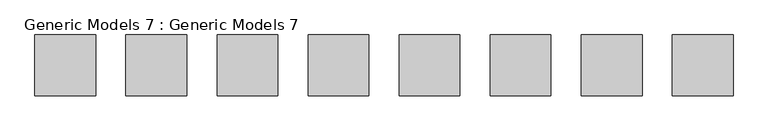
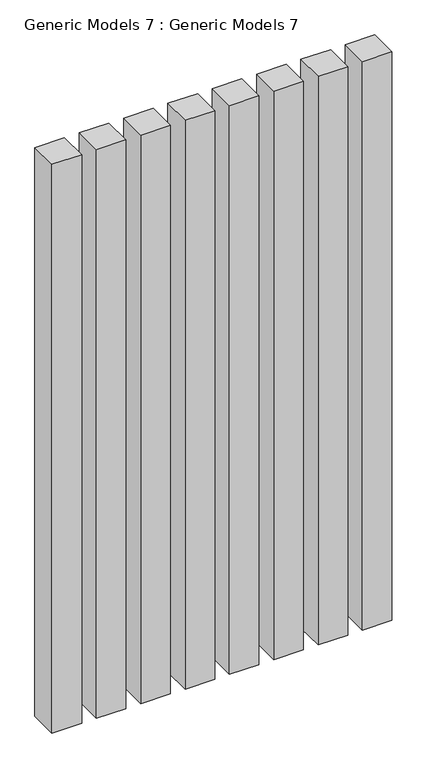
"""IFC4 building model written with IfcOpenShell, lengths in millimetres: proxy geometry, Generic Models 7 : Generic Models 7."""

from ifc_helpers import new_model, si_unit, frame, origin, place, context, project, spatial, polyline, outline, extrude, source, transform, mapped, element, save


def generic_models_7_generic_models_7_06f2fd99(model_context):
    return source(origin(), model_context, "Body", "SweptSolid", [
        extrude(outline(polyline([(-5066.7348456, -6024.70908), (-4914.3348456, -6024.70908), (-4914.3348456, -6177.10908), (-5066.7348456, -6177.10908), (-5066.7348456, -6024.70908)])), frame((0.0, 0.0, 3657.6), z_axis=(0.0, 0.0, 1.0), x_axis=(1.0, 0.0, 0.0)), (0.0, 0.0, 1.0), 3098.8),
        extrude(outline(polyline([(-4838.1348456, -6024.70908), (-4685.7348456, -6024.70908), (-4685.7348456, -6177.10908), (-4838.1348456, -6177.10908), (-4838.1348456, -6024.70908)])), frame((0.0, 0.0, 3657.6), z_axis=(0.0, 0.0, 1.0), x_axis=(1.0, 0.0, 0.0)), (0.0, 0.0, 1.0), 3098.8),
        extrude(outline(polyline([(-4609.5348456, -6024.70908), (-4457.1348456, -6024.70908), (-4457.1348456, -6177.10908), (-4609.5348456, -6177.10908), (-4609.5348456, -6024.70908)])), frame((0.0, 0.0, 3657.6), z_axis=(0.0, 0.0, 1.0), x_axis=(1.0, 0.0, 0.0)), (0.0, 0.0, 1.0), 3098.8),
        extrude(outline(polyline([(-4380.9348456, -6024.70908), (-4228.5348456, -6024.70908), (-4228.5348456, -6177.10908), (-4380.9348456, -6177.10908), (-4380.9348456, -6024.70908)])), frame((0.0, 0.0, 3657.6), z_axis=(0.0, 0.0, 1.0), x_axis=(1.0, 0.0, 0.0)), (0.0, 0.0, 1.0), 3098.8),
        extrude(outline(polyline([(-4152.3348456, -6024.70908), (-3999.9348456, -6024.70908), (-3999.9348456, -6177.10908), (-4152.3348456, -6177.10908), (-4152.3348456, -6024.70908)])), frame((0.0, 0.0, 3657.6), z_axis=(0.0, 0.0, 1.0), x_axis=(1.0, 0.0, 0.0)), (0.0, 0.0, 1.0), 3098.8),
        extrude(outline(polyline([(-3923.7348456, -6024.70908), (-3771.3348456, -6024.70908), (-3771.3348456, -6177.10908), (-3923.7348456, -6177.10908), (-3923.7348456, -6024.70908)])), frame((0.0, 0.0, 3657.6), z_axis=(0.0, 0.0, 1.0), x_axis=(1.0, 0.0, 0.0)), (0.0, 0.0, 1.0), 3098.8),
        extrude(outline(polyline([(-3695.1348456, -6024.70908), (-3542.7348456, -6024.70908), (-3542.7348456, -6177.10908), (-3695.1348456, -6177.10908), (-3695.1348456, -6024.70908)])), frame((0.0, 0.0, 3657.6), z_axis=(0.0, 0.0, 1.0), x_axis=(1.0, 0.0, 0.0)), (0.0, 0.0, 1.0), 3098.8),
        extrude(outline(polyline([(-3466.5348456, -6024.70908), (-3314.1348456, -6024.70908), (-3314.1348456, -6177.10908), (-3466.5348456, -6177.10908), (-3466.5348456, -6024.70908)])), frame((0.0, 0.0, 3657.6), z_axis=(0.0, 0.0, 1.0), x_axis=(1.0, 0.0, 0.0)), (0.0, 0.0, 1.0), 3098.8),
    ])


if __name__ == "__main__":
    model = new_model("IFC4")
    model_context = context("Model", 3, world=origin())
    ifc_project = project(units=[si_unit("LENGTHUNIT", "METRE", prefix="MILLI")], contexts=[model_context])
    site = spatial("IfcSite", under=ifc_project)
    building = spatial("IfcBuilding", under=site)
    placement = place(None, origin())
    generic_models_7_generic_models_7_shape = generic_models_7_generic_models_7_06f2fd99(model_context)
    element("IfcBuildingElementProxy", 1, Name="Generic Models 7 : Generic Models 7", ObjectType="Generic Models 7 : Generic Models 7", at=placement, inside=building, context=model_context, shape_type="MappedRepresentation", body=[
        mapped(generic_models_7_generic_models_7_shape, transform((0.0, 0.0, 0.0), x_axis=(1.0, 0.0, 0.0), y_axis=(0.0, 1.0, 0.0), z_axis=(0.0, 0.0, 1.0))),
    ])
    save(model, "model.ifc")

# Revit data of these elements
# Element 1 (IfcBuildingElementProxy, "Generic Models 7 : Generic Models 7")
#   Materials on its faces: "chocolate brown"
# Materials
#   "chocolate brown": class "Generic", colour RGB 120 120 120, transparency 0, Cost = 0
